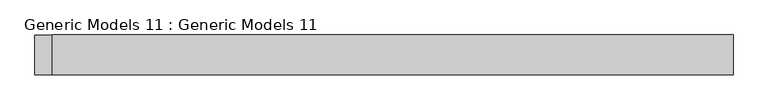
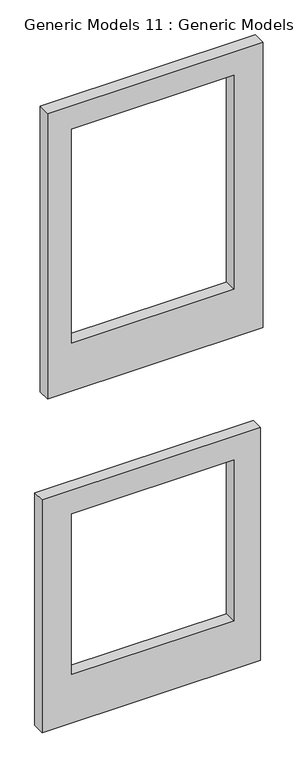
"""IFC4 building model written with IfcOpenShell, lengths in millimetres: proxy geometry, Generic Models 11 : Generic Models 11."""

from ifc_helpers import new_model, si_unit, frame, origin, place, context, project, spatial, polyline, outline, extrude, source, transform, mapped, element, save


def generic_models_11_generic_models_11_8cdfda78(model_context):
    return source(origin(), model_context, "Body", "SweptSolid", [
        extrude(outline(polyline([(5581.0228134, -9999.6996757), (5581.0228134, -11770.0991847), (3588.5355704, -11770.0991847), (3588.5355704, -9999.6996757), (5581.0228134, -9999.6996757)]), holes=[polyline([(5377.8228134, -10215.5695233), (4001.8016497, -10215.5695233), (4001.8016497, -11530.0195233), (5377.8228134, -11530.0195233), (5377.8228134, -10215.5695233)])]), frame((0.0, -14287.1752569, 0.0), z_axis=(0.0, 1.0, 0.0), x_axis=(0.0, 0.0, 1.0)), (0.0, 0.0, 1.0), 101.6),
        extrude(outline(polyline([(8875.941835, -9980.3565921), (8875.941835, -11725.9387656), (6429.1436541, -11725.9387656), (6429.1436541, -9980.3565921), (8875.941835, -9980.3565921)]), holes=[polyline([(8672.741835, -10215.5695233), (6841.9204311, -10215.5695233), (6841.9204311, -11530.0195233), (8672.741835, -11530.0195233), (8672.741835, -10215.5695233)])]), frame((0.0, -14287.1752569, 0.0), z_axis=(0.0, 1.0, 0.0), x_axis=(0.0, 0.0, 1.0)), (0.0, 0.0, 1.0), 101.6),
    ])


if __name__ == "__main__":
    model = new_model("IFC4")
    model_context = context("Model", 3, world=origin())
    ifc_project = project(units=[si_unit("LENGTHUNIT", "METRE", prefix="MILLI")], contexts=[model_context])
    site = spatial("IfcSite", under=ifc_project)
    building = spatial("IfcBuilding", under=site)
    placement = place(None, origin())
    generic_models_11_generic_models_11_shape = generic_models_11_generic_models_11_8cdfda78(model_context)
    element("IfcBuildingElementProxy", 1, Name="Generic Models 11 : Generic Models 11", ObjectType="Generic Models 11 : Generic Models 11", at=placement, inside=building, context=model_context, shape_type="MappedRepresentation", body=[
        mapped(generic_models_11_generic_models_11_shape, transform((0.0, 0.0, 0.0), x_axis=(1.0, 0.0, 0.0), y_axis=(0.0, 1.0, 0.0), z_axis=(0.0, 0.0, 1.0))),
    ])
    save(model, "model.ifc")
